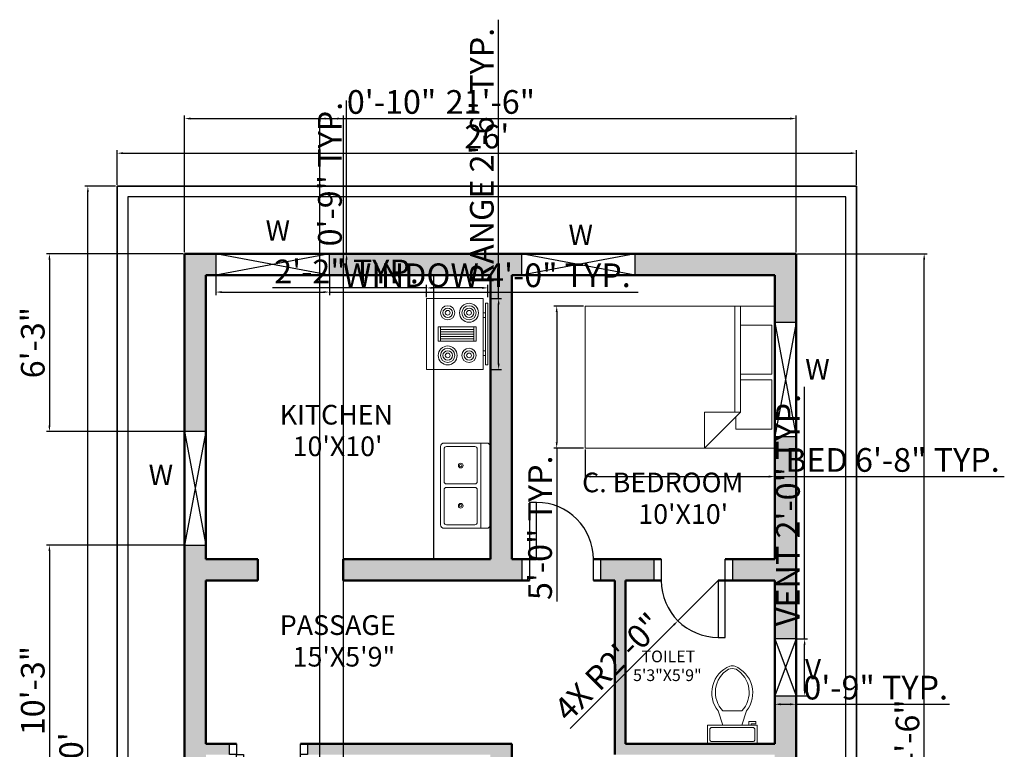
# Model space of a CAD drawing. Units: inches. Extents: x 2789 to 3623, y 2388 to 2993.
# Tile 2 of 5: x 2789 to 3205, y 2685 to 2993. Entities that reach past the tile are written whole.
import ezdxf

# ---------------------------------------------------------------- set-up
doc = ezdxf.new("R2010")
doc.units = ezdxf.units.IN
for name, color, linetype, lineweight in [('A-ANNO-DIMS', 2, 'Continuous', 18), ('A-ANNO-TEXT', 7, 'Continuous', 18), ('A-AREA-IDEN', 7, 'Continuous', 18), ('A-EQPM', 9, 'Continuous', 18), ('A-FLOR-CASE', 8, 'Continuous', 25), ('A-FLOR-FIXT', 9, 'Continuous', 18), ('A-FURN', 8, 'Continuous', 18), ('A-WALL', 7, 'Continuous', 50), ('A-WALL-PATT', 5, 'Continuous', 13), ('C-PROP', 7, 'Continuous', 35), ('d', 1, 'Continuous', 25), ('L-WALL', 7, 'Continuous', 25), ('v', 6, 'Continuous', 25), ('w', 170, 'Continuous', 25)]:
    doc.layers.add(name, color=color, linetype=linetype, lineweight=lineweight)
doc.styles.get("Standard").update_dxf_attribs({"font": 'arial.ttf'})
doc.dimstyles.new('ISO-25', dxfattribs={"dimtxt": 10, "dimasz": 2.5, "dimexe": 1.25, "dimexo": 0.625, "dimtad": 1, "dimlunit": 4, "dimtxsty": 'Standard', "dimcen": 2.5, "dimadec": 0, "dimazin": 0, "dimtfac": 1, "dimtmove": 0, "dimatfit": 3, "dimfxl": 1, "dimarcsym": 0})

# ---------------------------------------------------------------- blocks, each defined once
blk = doc.blocks.new('Range-Oven - 30 in top')
for p, q in [((0, -3), (30, -3)), ((12, -6), (18, -6)), ((13, -20), (13, -6)), ((14, -6), (14, -20)), ((15, -20), (15, -6)), ((16, -6), (16, -20)), ((17, -20), (17, -6)), ((18, -20), (12, -20)), ((6, -24), (6, -25)), ((8, -25), (8, -24)), ((22, -25), (22, -24)), ((24, -24), (24, -25))]:
    blk.add_line(p, q)
for points in [[(0, -24), (0, 0), (30, 0), (30, -24)], [(12, -21), (12, -5), (18, -5), (18, -21)], [(2, -26), (2, -25), (28, -25), (28, -26)]]:
    blk.add_lwpolyline(points, close=True)
for centre, radius in [((6, -9), 4), ((6, -9), 3), ((6, -9), 2), ((6, -9), 1), ((24, -9), 3), ((24, -9), 2), ((24, -9), 1), ((6, -18), 3), ((6, -18), 2), ((24, -18), 4), ((24, -18), 3), ((24, -18), 2), ((6, -18), 1), ((24, -18), 1)]:
    blk.add_circle(centre, radius)
blk = doc.blocks.new('Sink-double - 36 in top')
for p, q in [((-18, -4), (18, -4)), ((-0.75, -18.5), (-0.75, -6.5)), ((0.75, -6.5), (0.75, -18.5))]:
    blk.add_line(p, q)
for points in [[(-16.5, 0), (16.5, 0)], [(-18, -19.5), (-18, -1.5)], [(18, -1.5), (18, -19.5)], [(-16.5, -18.5), (-16.5, -6.5)], [(-15.5, -5.5), (-1.75, -5.5)], [(1.75, -5.5), (15.5, -5.5)], [(16.5, -6.5), (16.5, -18.5)], [(-1.75, -19.5), (-15.5, -19.5)], [(15.5, -19.5), (1.75, -19.5)], [(16.5, -21), (-16.5, -21)]]:
    blk.add_lwpolyline(points)
for centre, radius in [((-8.5, -12.5), 1), ((-8.5, -12.5), 0.5), ((8.5, -12.5), 1), ((8.5, -12.5), 0.5)]:
    blk.add_circle(centre, radius)
for centre, radius, start, end in [((-16.5, -1.5), 1.5, 90, 180), ((16.5, -1.5), 1.5, 0, 90), ((-15.5, -6.5), 1, 90, 180), ((-1.75, -6.5), 1, 0, 90), ((1.75, -6.5), 1, 90, 180), ((15.5, -6.5), 1, 0, 90), ((-16.5, -19.5), 1.5, 180, 270), ((-15.5, -18.5), 1, 180, 270), ((-1.75, -18.5), 1, 270, 0), ((1.75, -18.5), 1, 180, 270), ((15.5, -18.5), 1, 270, 0), ((16.5, -19.5), 1.5, 270, 0)]:
    blk.add_arc(centre, radius, start, end)
blk = doc.blocks.new('Toilet - top')
for p, q in [((9.5, -6), (9.5, -2)), ((-8, -8.5), (-8, -8)), ((-7, -8), (-7, -9.5)), ((-4, -8), (-6, -14)), ((4, -8), (6, -14)), ((-10, -8.5), (-8, -8.5)), ((-10, -9.5), (-10, -8.5)), ((-7, -9.5), (-10, -9.5)), ((4, -14), (-4, -14))]:
    blk.add_line(p, q)
blk.add_lwpolyline([(10.5, -8), (10.5, 0), (-10.5, 0), (-10.5, -8)], close=True)
for points in [[(-9.5, -2), (-9.5, -6)], [(8.5, -1), (-8.5, -1)], [(-8.5, -7), (8.5, -7)]]:
    blk.add_lwpolyline(points)
for centre, radius, start, end in [((-8.62, -1.88), 0.884, 81.8699, 188.1301), ((8.62, -1.88), 0.884, 351.8699, 98.1301), ((-8.62, -6.12), 0.884, 171.8699, 278.1301), ((8.62, -6.12), 0.884, 261.8699, 8.1301), ((3.52, -21.58), 12.17, 141.4691, 247.9714), ((4.2, -21.82), 11.33, 136.3677, 238.9468), ((-3.52, -21.58), 12.17, 292.0284, 38.5307), ((-4.2, -21.82), 11.33, 301.053, 43.6321), ((0, -27.88), 4, 245.7318, 294.2682), ((0, -29), 4, 254.8605, 285.1395)]:
    blk.add_arc(centre, radius, start, end)
blk = doc.blocks.new('Bed - Queen')
for p, q in [((0, -80.00003), (0, 0)), ((0, 0), (59.99999, 0)), ((59.99999, 0), (59.99999, -80.00003)), ((7.99999, -1.2), (28.79998, -1.2)), ((7.99999, -14.4), (7.99999, -1.2)), ((28.79998, -1.2), (28.79998, -14.4)), ((31.19999, -1.2), (51.99999, -1.2)), ((31.19999, -14.4), (31.19999, -1.2)), ((51.99999, -1.2), (51.99999, -16.4)), ((0, -14.4), (44.8, -14.4)), ((59.99999, -29.6), (44.8, -14.4)), ((44.8, -14.4), (44.8, -29.6)), ((51.99999, -16.4), (46.79936, -16.4)), ((44.8, -16.8), (0, -16.8)), ((44.8, -29.6), (59.99999, -29.6)), ((59.99999, -80.00003), (0, -80.00003))]:
    blk.add_line(p, q)
blk = doc.blocks.new('*D12')
at = {"layer": 'A-ANNO-DIMS', "color": 0, "lineweight": -2, "transparency": 16777216}
for p, q in [((2830.55, 2923.47), (2830.55, 2938.03)), ((3142.55, 2923.47), (3142.55, 2938.03)), ((2833.05, 2936.78), (3140.05, 2936.78))]:
    blk.add_line(p, q, dxfattribs=at)
at = {"layer": 'A-ANNO-DIMS', "color": 0, "transparency": 16777216}
for points in [[(2833.05, 2937.19), (2833.05, 2936.36), (2830.55, 2936.78)], [(3140.05, 2937.19), (3140.05, 2936.36), (3142.55, 2936.78)]]:
    blk.add_solid(points, dxfattribs=at)
at = {"layer": 'Defpoints', "color": 0, "transparency": 16777216}
for p in [(3142.55, 2936.78), (2830.55, 2922.84), (3142.55, 2922.84)]:
    blk.add_point(p, dxfattribs=at)
at = {"layer": 'A-ANNO-DIMS', "color": 0, "transparency": 16777216, "insert": (2986.55, 2942.51), "char_height": 10, "attachment_point": 5}
blk.add_mtext("26'", dxfattribs=at)
blk = doc.blocks.new('*D13')
at = {"layer": 'A-ANNO-DIMS', "color": 0, "lineweight": -2, "transparency": 16777216}
for p, q in [((2829.92, 2922.84), (2816.96, 2922.84)), ((2818.21, 2445.34), (2818.21, 2920.34)), ((2829.92, 2442.84), (2816.96, 2442.84))]:
    blk.add_line(p, q, dxfattribs=at)
at = {"layer": 'A-ANNO-DIMS', "color": 0, "transparency": 16777216}
for points in [[(2817.8, 2920.34), (2818.63, 2920.34), (2818.21, 2922.84)], [(2817.8, 2445.34), (2818.63, 2445.34), (2818.21, 2442.84)]]:
    blk.add_solid(points, dxfattribs=at)
at = {"layer": 'Defpoints', "color": 0, "transparency": 16777216}
for p in [(2818.21, 2922.84), (2830.55, 2922.84), (2830.55, 2442.84)]:
    blk.add_point(p, dxfattribs=at)
at = {"layer": 'A-ANNO-DIMS', "color": 0, "transparency": 16777216, "insert": (2812.48, 2682.84), "char_height": 10, "attachment_point": 5, "rotation": 90}
blk.add_mtext("40'", dxfattribs=at)
blk = doc.blocks.new('DOOR-24IN-JAMB-9IN')
for points in [[(0, 24), (-3, 24), (-3, 0), (0, 0)], [(-6, 0), (-3, 0), (-3, -9), (-6, -9)], [(24, 0), (27, 0), (27, -9), (24, -9)]]:
    blk.add_lwpolyline(points, close=True)
blk.add_arc((0, 0), 24, 0, 90)
blk = doc.blocks.new('DOOR-24IN-JAMB-4_5IN')
for points in [[(-3, 0), (-6, 0), (-6, 4.5), (-3, 4.5)], [(27, 0), (24, 0), (24, 4.5), (27, 4.5)], [(0, -24), (-3, -24), (-3, 0), (0, 0)]]:
    blk.add_lwpolyline(points, close=True)
blk.add_arc((0, 0), 24, 270, 0)
blk = doc.blocks.new('WINDOW-48IN')
for p, q in [((48, 9), (0, 0)), ((48, 0), (0, 9))]:
    blk.add_line(p, q)
blk.add_lwpolyline([(0, 9), (0, 0), (48, 0), (48, 9)], close=True)
blk = doc.blocks.new('VENT-24IN')
for p, q in [((0, 24), (9, 0)), ((9, 24), (0, 0))]:
    blk.add_line(p, q)
blk.add_lwpolyline([(0, 0), (9, 0), (9, 24), (0, 24)], close=True)
blk = doc.blocks.new('*D20')
at = {"layer": 'A-ANNO-DIMS', "color": 0, "lineweight": -2, "transparency": 16777216}
for p, q in [((2872.18, 2884.72), (2872.18, 2876.89)), ((2920.18, 2884.72), (2920.18, 2876.89)), ((2874.68, 2878.14), (2917.68, 2878.14)), ((2920.18, 2878.14), (3050.48, 2878.14))]:
    blk.add_line(p, q, dxfattribs=at)
at = {"layer": 'A-ANNO-DIMS', "color": 0, "transparency": 16777216}
for points in [[(2874.68, 2878.56), (2874.68, 2877.73), (2872.18, 2878.14)], [(2917.68, 2878.56), (2917.68, 2877.73), (2920.18, 2878.14)]]:
    blk.add_solid(points, dxfattribs=at)
at = {"layer": 'Defpoints', "color": 0, "transparency": 16777216}
for p in [(2872.18, 2885.34), (2920.18, 2885.34), (2920.18, 2878.14)]:
    blk.add_point(p, dxfattribs=at)
at = {"layer": 'A-ANNO-DIMS', "color": 0, "transparency": 16777216, "insert": (2986.58, 2883.94), "char_height": 10, "attachment_point": 5}
blk.add_mtext('WINDOW 4\'-0" TYP.', dxfattribs=at)
blk = doc.blocks.new('*D21')
at = {"layer": 'A-ANNO-DIMS', "color": 0, "lineweight": -2, "transparency": 16777216}
for p, q in [((2927.38, 2894.34), (2927.38, 2959.05)), ((2920.81, 2894.34), (2928.63, 2894.34)), ((2927.38, 2887.84), (2927.38, 2891.84)), ((2920.81, 2885.34), (2928.63, 2885.34))]:
    blk.add_line(p, q, dxfattribs=at)
at = {"layer": 'A-ANNO-DIMS', "color": 0, "transparency": 16777216}
for points in [[(2926.97, 2891.84), (2927.8, 2891.84), (2927.38, 2894.34)], [(2926.97, 2887.84), (2927.8, 2887.84), (2927.38, 2885.34)]]:
    blk.add_solid(points, dxfattribs=at)
at = {"layer": 'Defpoints', "color": 0, "transparency": 16777216}
for p in [(2920.18, 2894.34), (2927.38, 2894.34), (2920.18, 2885.34)]:
    blk.add_point(p, dxfattribs=at)
at = {"layer": 'A-ANNO-DIMS', "color": 0, "transparency": 16777216, "insert": (2921.65, 2927.94), "char_height": 10, "attachment_point": 5, "rotation": 90}
blk.add_mtext('0\'-9" TYP.', dxfattribs=at)
blk = doc.blocks.new('*D24')
at = {"layer": 'A-ANNO-DIMS', "color": 0, "lineweight": -2, "transparency": 16777216}
for p, q in [((3028.05, 2811.61), (3028.05, 2798.99)), ((3108.05, 2811.61), (3108.05, 2798.99)), ((3030.55, 2800.24), (3105.55, 2800.24)), ((3108.05, 2800.24), (3204.92, 2800.24))]:
    blk.add_line(p, q, dxfattribs=at)
at = {"layer": 'A-ANNO-DIMS', "color": 0, "transparency": 16777216}
for points in [[(3030.55, 2800.66), (3030.55, 2799.82), (3028.05, 2800.24)], [(3105.55, 2800.66), (3105.55, 2799.82), (3108.05, 2800.24)]]:
    blk.add_solid(points, dxfattribs=at)
at = {"layer": 'Defpoints', "color": 0, "transparency": 16777216}
for p in [(3028.05, 2812.24), (3108.05, 2812.24), (3108.05, 2800.24)]:
    blk.add_point(p, dxfattribs=at)
at = {"layer": 'A-ANNO-DIMS', "color": 0, "transparency": 16777216, "insert": (3157.73, 2805.97), "char_height": 10, "attachment_point": 5}
blk.add_mtext('BED 6\'-8" TYP.', dxfattribs=at)
blk = doc.blocks.new('*D25')
at = {"layer": 'A-ANNO-DIMS', "color": 0, "lineweight": -2, "transparency": 16777216}
for p, q in [((3027.42, 2872.24), (3014.8, 2872.24)), ((3016.05, 2869.74), (3016.05, 2814.74)), ((3027.42, 2812.24), (3014.8, 2812.24)), ((3016.05, 2812.24), (3016.05, 2747.53))]:
    blk.add_line(p, q, dxfattribs=at)
at = {"layer": 'A-ANNO-DIMS', "color": 0, "transparency": 16777216}
for points in [[(3015.63, 2869.74), (3016.46, 2869.74), (3016.05, 2872.24)], [(3015.63, 2814.74), (3016.46, 2814.74), (3016.05, 2812.24)]]:
    blk.add_solid(points, dxfattribs=at)
at = {"layer": 'Defpoints', "color": 0, "transparency": 16777216}
for p in [(3028.05, 2872.24), (3016.05, 2812.24), (3028.05, 2812.24)]:
    blk.add_point(p, dxfattribs=at)
at = {"layer": 'A-ANNO-DIMS', "color": 0, "transparency": 16777216, "insert": (3010.32, 2778.64), "char_height": 10, "attachment_point": 5, "rotation": 90}
blk.add_mtext('5\'-0" TYP.', dxfattribs=at)
blk = doc.blocks.new('*D28')
at = {"layer": 'A-ANNO-DIMS', "color": 0, "lineweight": -2, "transparency": 16777216}
for p, q in [((2991.55, 2875.4), (2991.55, 2993.15)), ((2987.67, 2875.4), (2992.8, 2875.4)), ((2991.55, 2847.9), (2991.55, 2872.9)), ((2987.67, 2845.4), (2992.8, 2845.4))]:
    blk.add_line(p, q, dxfattribs=at)
at = {"layer": 'A-ANNO-DIMS', "color": 0, "transparency": 16777216}
for points in [[(2991.13, 2872.9), (2991.96, 2872.9), (2991.55, 2875.4)], [(2991.13, 2847.9), (2991.96, 2847.9), (2991.55, 2845.4)]]:
    blk.add_solid(points, dxfattribs=at)
at = {"layer": 'Defpoints', "color": 0, "transparency": 16777216}
for p in [(2987.05, 2875.4), (2991.55, 2875.4), (2987.05, 2845.4)]:
    blk.add_point(p, dxfattribs=at)
at = {"layer": 'A-ANNO-DIMS', "color": 0, "transparency": 16777216, "insert": (2985.75, 2935.53), "char_height": 10, "attachment_point": 5, "rotation": 90}
blk.add_mtext('RANGE 2\'-6" TYP.', dxfattribs=at)
blk = doc.blocks.new('*D29')
at = {"layer": 'A-ANNO-DIMS', "color": 0, "lineweight": -2, "transparency": 16777216}
for p, q in [((2961.05, 2879.9), (2896.17, 2879.9)), ((2961.05, 2876.03), (2961.05, 2881.15)), ((2984.55, 2879.9), (2963.55, 2879.9)), ((2987.05, 2876.03), (2987.05, 2881.15))]:
    blk.add_line(p, q, dxfattribs=at)
at = {"layer": 'A-ANNO-DIMS', "color": 0, "transparency": 16777216}
for points in [[(2963.55, 2880.32), (2963.55, 2879.49), (2961.05, 2879.9)], [(2984.55, 2880.32), (2984.55, 2879.49), (2987.05, 2879.9)]]:
    blk.add_solid(points, dxfattribs=at)
at = {"layer": 'Defpoints', "color": 0, "transparency": 16777216}
for p in [(2961.05, 2879.9), (2961.05, 2875.4), (2987.05, 2875.4)]:
    blk.add_point(p, dxfattribs=at)
at = {"layer": 'A-ANNO-DIMS', "color": 0, "transparency": 16777216, "insert": (2927.36, 2885.55), "char_height": 10, "attachment_point": 5}
blk.add_mtext('2\'-2" TYP.', dxfattribs=at)
blk = doc.blocks.new('*D40')
at = {"layer": 'A-ANNO-DIMS', "color": 0, "lineweight": -2, "transparency": 16777216}
for p, q in [((3120.65, 2731.71), (3120.65, 2838.07)), ((3117.67, 2731.71), (3121.9, 2731.71)), ((3120.65, 2710.21), (3120.65, 2729.21)), ((3117.67, 2707.71), (3121.9, 2707.71))]:
    blk.add_line(p, q, dxfattribs=at)
at = {"layer": 'A-ANNO-DIMS', "color": 0, "transparency": 16777216}
for points in [[(3120.23, 2729.21), (3121.06, 2729.21), (3120.65, 2731.71)], [(3120.23, 2710.21), (3121.06, 2710.21), (3120.65, 2707.71)]]:
    blk.add_solid(points, dxfattribs=at)
at = {"layer": 'Defpoints', "color": 0, "transparency": 16777216}
for p in [(3117.05, 2731.71), (3120.65, 2731.71), (3117.05, 2707.71)]:
    blk.add_point(p, dxfattribs=at)
at = {"layer": 'A-ANNO-DIMS', "color": 0, "transparency": 16777216, "insert": (3114.92, 2786.14), "char_height": 10, "attachment_point": 5, "rotation": 90}
blk.add_mtext('VENT 2\'-0" TYP.', dxfattribs=at)
blk = doc.blocks.new('*D41')
at = {"layer": 'A-ANNO-DIMS', "color": 0, "lineweight": -2, "transparency": 16777216}
for p, q in [((3108.05, 2707.09), (3108.05, 2702.86)), ((3117.05, 2707.09), (3117.05, 2702.86)), ((3110.55, 2704.11), (3114.55, 2704.11)), ((3117.05, 2704.11), (3181.75, 2704.11))]:
    blk.add_line(p, q, dxfattribs=at)
at = {"layer": 'A-ANNO-DIMS', "color": 0, "transparency": 16777216}
for points in [[(3110.55, 2704.53), (3110.55, 2703.69), (3108.05, 2704.11)], [(3114.55, 2704.53), (3114.55, 2703.69), (3117.05, 2704.11)]]:
    blk.add_solid(points, dxfattribs=at)
at = {"layer": 'Defpoints', "color": 0, "transparency": 16777216}
for p in [(3108.05, 2707.71), (3117.05, 2707.71), (3117.05, 2704.11)]:
    blk.add_point(p, dxfattribs=at)
at = {"layer": 'A-ANNO-DIMS', "color": 0, "transparency": 16777216, "insert": (3150.65, 2709.84), "char_height": 10, "attachment_point": 5}
blk.add_mtext('0\'-9" TYP.', dxfattribs=at)
blk = doc.blocks.new('*D42')
at = {"layer": 'A-ANNO-DIMS', "color": 0, "lineweight": -2, "transparency": 16777216}
for p, q in [((2859.05, 2894.97), (2859.05, 2952.64)), ((2861.55, 2951.39), (3114.55, 2951.39)), ((3117.05, 2894.97), (3117.05, 2952.64))]:
    blk.add_line(p, q, dxfattribs=at)
at = {"layer": 'A-ANNO-DIMS', "color": 0, "transparency": 16777216}
for points in [[(2861.55, 2951.81), (2861.55, 2950.98), (2859.05, 2951.39)], [(3114.55, 2951.81), (3114.55, 2950.98), (3117.05, 2951.39)]]:
    blk.add_solid(points, dxfattribs=at)
at = {"layer": 'Defpoints', "color": 0, "transparency": 16777216}
for p in [(3117.05, 2951.39), (2859.05, 2894.34), (3117.05, 2894.34)]:
    blk.add_point(p, dxfattribs=at)
at = {"layer": 'A-ANNO-DIMS', "color": 0, "transparency": 16777216, "insert": (2988.05, 2957.12), "char_height": 10, "attachment_point": 5}
blk.add_mtext('21\'-6"', dxfattribs=at)
blk = doc.blocks.new('*D43')
at = {"layer": 'A-ANNO-DIMS', "color": 0, "lineweight": -2, "transparency": 16777216}
for p, q in [((3117.67, 2894.34), (3172.35, 2894.34)), ((3171.1, 2482.84), (3171.1, 2891.84)), ((3117.67, 2480.34), (3172.35, 2480.34))]:
    blk.add_line(p, q, dxfattribs=at)
at = {"layer": 'A-ANNO-DIMS', "color": 0, "transparency": 16777216}
for points in [[(3170.68, 2891.84), (3171.51, 2891.84), (3171.1, 2894.34)], [(3170.68, 2482.84), (3171.51, 2482.84), (3171.1, 2480.34)]]:
    blk.add_solid(points, dxfattribs=at)
at = {"layer": 'Defpoints', "color": 0, "transparency": 16777216}
for p in [(3117.05, 2894.34), (3171.1, 2894.34), (3117.05, 2480.34)]:
    blk.add_point(p, dxfattribs=at)
at = {"layer": 'A-ANNO-DIMS', "color": 0, "transparency": 16777216, "insert": (3165.36, 2687.34), "char_height": 10, "attachment_point": 5, "rotation": 90}
blk.add_mtext('34\'-6"', dxfattribs=at)
blk = doc.blocks.new('*D48')
at = {"layer": 'A-ANNO-DIMS', "color": 0, "lineweight": -2, "transparency": 16777216}
for p, q in [((2916.05, 2520.72), (2916.05, 2952.64)), ((2918.55, 2951.39), (2923.55, 2951.39)), ((2926.05, 2520.72), (2926.05, 2952.64)), ((2926.05, 2951.39), (2964.15, 2951.39))]:
    blk.add_line(p, q, dxfattribs=at)
at = {"layer": 'A-ANNO-DIMS', "color": 0, "transparency": 16777216}
for points in [[(2918.55, 2951.81), (2918.55, 2950.98), (2916.05, 2951.39)], [(2923.55, 2951.81), (2923.55, 2950.98), (2926.05, 2951.39)]]:
    blk.add_solid(points, dxfattribs=at)
at = {"layer": 'Defpoints', "color": 0, "transparency": 16777216}
for p in [(2926.05, 2951.39), (2916.05, 2520.09), (2926.05, 2520.09)]:
    blk.add_point(p, dxfattribs=at)
at = {"layer": 'A-ANNO-DIMS', "color": 0, "transparency": 16777216, "insert": (2946.35, 2957.12), "char_height": 10, "attachment_point": 5}
blk.add_mtext('0\'-10"', dxfattribs=at)
blk = doc.blocks.new('*D52')
at = {"layer": 'A-ANNO-DIMS', "color": 0, "lineweight": -2, "transparency": 16777216}
for p, q in [((2858.42, 2894.34), (2800.75, 2894.34)), ((2802, 2891.84), (2802, 2821.77)), ((2858.42, 2819.27), (2800.75, 2819.27))]:
    blk.add_line(p, q, dxfattribs=at)
at = {"layer": 'A-ANNO-DIMS', "color": 0, "transparency": 16777216}
for points in [[(2801.58, 2891.84), (2802.41, 2891.84), (2802, 2894.34)], [(2801.58, 2821.77), (2802.41, 2821.77), (2802, 2819.27)]]:
    blk.add_solid(points, dxfattribs=at)
at = {"layer": 'Defpoints', "color": 0, "transparency": 16777216}
for p in [(2859.05, 2894.34), (2802, 2819.27), (2859.05, 2819.27)]:
    blk.add_point(p, dxfattribs=at)
at = {"layer": 'A-ANNO-DIMS', "color": 0, "transparency": 16777216, "insert": (2796.26, 2856.8), "char_height": 10, "attachment_point": 5, "rotation": 90}
blk.add_mtext('6\'-3"', dxfattribs=at)
blk = doc.blocks.new('*D53')
at = {"layer": 'A-ANNO-DIMS', "color": 0, "lineweight": -2, "transparency": 16777216}
for p, q in [((2858.42, 2771.27), (2800.75, 2771.27)), ((2802, 2768.77), (2802, 2651.02)), ((2858.42, 2648.52), (2800.75, 2648.52))]:
    blk.add_line(p, q, dxfattribs=at)
at = {"layer": 'A-ANNO-DIMS', "color": 0, "transparency": 16777216}
for points in [[(2801.58, 2768.77), (2802.41, 2768.77), (2802, 2771.27)], [(2801.58, 2651.02), (2802.41, 2651.02), (2802, 2648.52)]]:
    blk.add_solid(points, dxfattribs=at)
at = {"layer": 'Defpoints', "color": 0, "transparency": 16777216}
for p in [(2859.05, 2771.27), (2802, 2648.52), (2859.05, 2648.52)]:
    blk.add_point(p, dxfattribs=at)
at = {"layer": 'A-ANNO-DIMS', "color": 0, "transparency": 16777216, "insert": (2796.26, 2709.89), "char_height": 10, "attachment_point": 5, "rotation": 90}
blk.add_mtext('10\'-3"', dxfattribs=at)
blk = doc.blocks.new('*D59')
at = {"layer": 'A-ANNO-DIMS', "color": 0, "lineweight": -2, "transparency": 16777216}
for p, q in [((3084.18, 2756.34), (3067.21, 2739.37)), ((3021.75, 2693.91), (3065.44, 2737.6))]:
    blk.add_line(p, q, dxfattribs=at)
at = {"layer": 'A-ANNO-DIMS', "color": 0, "transparency": 16777216}
blk.add_solid([(3065.15, 2737.9), (3065.74, 2737.31), (3067.21, 2739.37)], dxfattribs=at)
at = {"layer": 'Defpoints', "color": 0, "transparency": 16777216}
for p in [(3084.18, 2756.34), (3067.21, 2739.37)]:
    blk.add_point(p, dxfattribs=at)
at = {"layer": 'A-ANNO-DIMS', "color": 0, "transparency": 16777216, "insert": (3038.66, 2718.92), "char_height": 10, "attachment_point": 5, "rotation": 45.0007}
blk.add_mtext('4X R2\'-0"', dxfattribs=at)

msp = doc.modelspace()

# ---------------------------------------------------------------- hatches: boundary and pattern name
at = {"layer": 'A-WALL-PATT'}
h = msp.add_hatch(color=256, dxfattribs=at)
h.dxf.hatch_style = 1
h.paths.add_polyline_path([(2868.048, 2600.516), (2859.048, 2600.516), (2859.048, 2480.342), (2996.048, 2480.342), (2996.048, 2489.342), (2868.048, 2489.342), (2868.048, 2553.842), (3004.548, 2553.842), (3004.548, 2562.842), (2997.048, 2562.842), (2997.048, 2687.342), (2910.917, 2687.342), (2910.917, 2682.842), (2988.048, 2682.842), (2988.048, 2562.842), (2868.048, 2562.842)])
h.paths.add_polyline_path([(2996.048, 2523.092), (2916.048, 2523.092), (2916.048, 2520.092), (2996.048, 2520.092)], flags=17)
h.paths.add_polyline_path([(3065.118, 2562.842), (3052.548, 2562.842), (3052.548, 2553.842), (3065.118, 2553.842)])
h.paths.add_polyline_path([(3117.048, 2569.319), (3108.048, 2569.319), (3108.048, 2562.842), (3098.118, 2562.842), (3098.118, 2553.842), (3117.048, 2553.842)])
h.paths.add_polyline_path([(3117.048, 2707.71), (3108.048, 2707.71), (3108.048, 2687.342), (3045.048, 2687.342), (3045.048, 2756.342), (3057.181, 2756.342), (3057.181, 2765.342), (3034.539, 2765.342), (3034.539, 2756.342), (3040.548, 2756.342), (3040.548, 2682.842), (3108.048, 2682.842), (3108.048, 2617.319), (3117.048, 2617.319)])
h.paths.add_polyline_path([(3117.048, 2817.229), (3108.048, 2817.229), (3108.048, 2812.239), (3108.048, 2765.342), (3090.181, 2765.342), (3090.181, 2756.342), (3108.048, 2756.342), (3108.048, 2731.71), (3117.048, 2731.71)])
h.paths.add_polyline_path([(2868.048, 2682.842), (2877.917, 2682.842), (2877.917, 2687.342), (2868.048, 2687.342), (2868.048, 2756.342), (2889.977, 2756.342), (2889.977, 2765.342), (2868.048, 2765.342), (2868.048, 2771.267), (2859.048, 2771.267), (2859.048, 2648.516), (2868.048, 2648.516)])
h.paths.add_polyline_path([(3001.539, 2765.342), (2997.048, 2765.342), (2997.048, 2885.342), (3001.182, 2885.342), (3001.182, 2894.342), (2920.184, 2894.342), (2920.184, 2885.342), (2988.048, 2885.342), (2988.048, 2765.342), (2925.977, 2765.342), (2925.977, 2756.342), (3001.539, 2756.342)])
h.paths.add_polyline_path([(2868.048, 2885.342), (2872.184, 2885.342), (2872.184, 2894.342), (2859.048, 2894.342), (2859.048, 2819.267), (2868.048, 2819.267)])
h.paths.add_polyline_path([(3117.048, 2894.342), (3049.182, 2894.342), (3049.182, 2885.342), (3108.048, 2885.342), (3108.048, 2865.229), (3117.048, 2865.229)])
h.paths.add_polyline_path([(3025.421, 2540.366), (3041.067, 2540.366), (3041.067, 2553.271), (3025.421, 2553.271)], flags=9)
h.paths.add_polyline_path([(3118.771, 2839.078), (3134.416, 2839.078), (3134.416, 2851.983), (3118.771, 2851.983)], flags=9)
h.paths.add_polyline_path([(3118.682, 2712.44), (3131, 2712.44), (3131, 2725.345), (3118.682, 2725.345)], flags=9)
h.paths.add_polyline_path([(3118.47, 2582.859), (3134.115, 2582.859), (3134.115, 2595.763), (3118.47, 2595.763)], flags=9)
h.paths.add_polyline_path([(2842.843, 2619.924), (2858.489, 2619.924), (2858.489, 2632.829), (2842.843, 2632.829)], flags=9)
h.paths.add_polyline_path([(2841.723, 2794.475), (2857.368, 2794.475), (2857.368, 2807.38), (2841.723, 2807.38)], flags=9)
h.paths.add_polyline_path([(3018.872, 2895.803), (3034.517, 2895.803), (3034.517, 2908.708), (3018.872, 2908.708)], flags=9)
h.paths.add_polyline_path([(2891.065, 2897.701), (2906.71, 2897.701), (2906.71, 2910.606), (2891.065, 2910.606)], flags=9)
h.paths.add_polyline_path([(2898.76, 2503.274), (2898.76, 2543.14), (2886.045, 2543.14), (2886.045, 2503.274)], flags=25)
h.paths.add_polyline_path([(2885.453, 2497.829), (2885.453, 2542.718), (2872.568, 2542.718), (2872.568, 2497.829)], flags=25)
h.paths.add_polyline_path([(3033.853, 2492.441), (3086.618, 2492.441), (3086.618, 2505.156), (3033.853, 2505.156)], flags=9)
h.paths.add_polyline_path([(3039.46, 2505.748), (3086.274, 2505.748), (3086.274, 2518.633), (3039.46, 2518.633)], flags=9)
h.paths.add_polyline_path([(3048.345, 2778.023), (3090.544, 2778.023), (3090.544, 2790.738), (3048.345, 2790.738)], flags=9)
h.paths.add_polyline_path([(3024.618, 2791.33), (3106.873, 2791.33), (3106.873, 2804.214), (3024.618, 2804.214)], flags=9)
h.paths.add_polyline_path([(3047.007, 2712.567), (3076.988, 2712.567), (3076.988, 2720.13), (3047.007, 2720.13)], flags=25)
h.paths.add_polyline_path([(3050.563, 2720.481), (3079.162, 2720.481), (3079.162, 2728.14), (3050.563, 2728.14)], flags=25)
h.paths.add_polyline_path([(3000.345, 2609.496), (3042.544, 2609.496), (3042.544, 2622.211), (3000.345, 2622.211)], flags=9)
h.paths.add_polyline_path([(3001.972, 2623.016), (3035.131, 2623.016), (3035.131, 2635.468), (3001.972, 2635.468)], flags=9)
h.paths.add_polyline_path([(2910.315, 2645.374), (2952.514, 2645.374), (2952.514, 2658.089), (2910.315, 2658.089)], flags=25)
h.paths.add_polyline_path([(2904.87, 2658.68), (2985.189, 2658.68), (2985.189, 2671.565), (2904.87, 2671.565)], flags=25)
h.paths.add_polyline_path([(2902.494, 2717.778), (2948.81, 2717.778), (2948.81, 2730.493), (2902.494, 2730.493)], flags=9)
h.paths.add_polyline_path([(2897.051, 2731.086), (2956.772, 2731.086), (2956.772, 2743.962), (2897.051, 2743.962)], flags=9)
h.paths.add_polyline_path([(2902.494, 2806.621), (2944.693, 2806.621), (2944.693, 2819.336), (2902.494, 2819.336)], flags=9)
h.paths.add_polyline_path([(2897.051, 2819.929), (2955.464, 2819.929), (2955.464, 2832.806), (2897.051, 2832.806)], flags=9)

# ---------------------------------------------------------------- linework, layer by layer
at = {"layer": 'A-FLOR-CASE'}
msp.add_line((2964.048, 2885.342), (2964.048, 2765.342), dxfattribs=at)
at = {"layer": 'A-WALL'}
for p, q in [((2859.048, 2894.342), (2859.048, 2480.342)), ((3117.048, 2894.342), (2859.048, 2894.342)), ((3117.048, 2553.842), (3117.048, 2894.342)), ((2868.048, 2885.342), (2868.048, 2765.342)), ((2988.048, 2885.342), (2868.048, 2885.342)), ((2988.048, 2885.342), (2988.048, 2765.342)), ((3108.048, 2885.342), (2997.048, 2885.342)), ((2997.048, 2885.342), (2997.048, 2765.342)), ((3108.048, 2765.342), (3108.048, 2885.342)), ((2889.977, 2765.342), (2868.048, 2765.342)), ((2889.977, 2756.342), (2889.977, 2765.342)), ((2988.048, 2765.342), (2925.977, 2765.342)), ((2925.977, 2756.342), (2925.977, 2765.342)), ((3007.539, 2765.342), (2997.048, 2765.342)), ((3060.181, 2765.342), (3031.539, 2765.342)), ((3108.048, 2765.342), (3087.181, 2765.342)), ((2868.048, 2756.342), (2868.048, 2687.342)), ((2889.977, 2756.342), (2868.048, 2756.342)), ((3004.539, 2756.342), (2925.977, 2756.342)), ((3040.548, 2756.342), (3031.539, 2756.342)), ((3040.548, 2682.842), (3040.548, 2756.342)), ((3045.048, 2687.342), (3045.048, 2756.342)), ((3060.181, 2756.342), (3045.048, 2756.342)), ((3108.048, 2756.342), (3084.181, 2756.342)), ((3108.048, 2687.342), (3108.048, 2756.342)), ((2880.917, 2687.342), (2868.048, 2687.342)), ((2997.048, 2687.342), (2907.917, 2687.342)), ((2997.048, 2687.342), (2997.048, 2562.842)), ((3108.048, 2687.342), (3045.048, 2687.342))]:
    msp.add_line(p, q, dxfattribs=at)
at = {"layer": 'C-PROP'}
msp.add_lwpolyline([(2830.548, 2442.842), (3142.548, 2442.842), (3142.548, 2922.842), (2830.548, 2922.842)], close=True, dxfattribs=at)
at = {"layer": 'L-WALL'}
for p, q in [((3138.048, 2918.342), (2835.048, 2918.342)), ((2835.048, 2918.342), (2835.048, 2447.342)), ((3138.048, 2447.342), (3138.048, 2918.342))]:
    msp.add_line(p, q, dxfattribs=at)

# ---------------------------------------------------------------- block references
at = {"layer": 'A-EQPM', "rotation": 90}
msp.add_blockref('Range-Oven - 30 in top', (2961.048, 2845.404), dxfattribs=at)
at = {"layer": 'A-FLOR-FIXT'}
for name, p, rotation in [('Sink-double - 36 in top', (2988.048, 2796.411), 270), ('Toilet - top', (3090.13, 2687.342), 180)]:
    msp.add_blockref(name, p, dxfattribs=dict(at, rotation=rotation))
at = {"layer": 'A-FURN', "rotation": 270}
msp.add_blockref('Bed - Queen', (3108.048, 2872.239), dxfattribs=at)
at = {"layer": 'd'}
for name, p in [('DOOR-24IN-JAMB-9IN', (3007.539, 2765.342)), ('DOOR-24IN-JAMB-4_5IN', (2883.917, 2682.842))]:
    msp.add_blockref(name, p, dxfattribs=at)
at = {"layer": 'd', "rotation": 180}
msp.add_blockref('DOOR-24IN-JAMB-9IN', (3084.181, 2756.342), dxfattribs=at)
at = {"layer": 'v'}
msp.add_blockref('VENT-24IN', (3108.048, 2707.71), dxfattribs=at)
at = {"layer": 'w'}
for p in [(2872.184, 2885.342), (3001.182, 2885.342)]:
    msp.add_blockref('WINDOW-48IN', p, dxfattribs=at)
at = {"layer": 'w', "rotation": 90.00000000000036}
for p in [(3117.048, 2817.229), (2868.048, 2771.267)]:
    msp.add_blockref('WINDOW-48IN', p, dxfattribs=at)

# ---------------------------------------------------------------- texts
at = {"layer": 'A-ANNO-TEXT'}
for s, p in [('W', (2893.216, 2899.852)), ('W', (3021.023, 2897.954)), ('W', (3120.922, 2841.229)), ('W', (2843.874, 2796.626)), ('V', (3120.833, 2714.591))]:
    msp.add_text(s, height=8.603, dxfattribs=at).set_placement(p)
at = {"layer": 'A-AREA-IDEN'}
for s, height, p in [('KITCHEN ', 8.3011, (2899.197, 2822.217)), ("10'X10'", 8.3011, (2904.613, 2808.882)), ('C. BEDROOM ', 8.30108, (3026.765, 2793.619)), ("10'X10'", 8.3011, (3050.465, 2780.284)), ('PASSAGE', 8.3011, (2899.197, 2733.374)), ('15\'X5\'9"', 8.3011, (2904.613, 2720.039)), ('TOILET ', 4.9345, (3051.839, 2721.842)), ('5\'3"X5\'9"', 4.9345, (3048.268, 2713.915))]:
    msp.add_text(s, height=height, dxfattribs=at).set_placement(p)

# ---------------------------------------------------------------- dimensions: what is measured, and where the dimension line sits
at = {"layer": 'A-ANNO-DIMS'}
for base, p1, p2, angle, text, picture, middle in [((2991.548, 2875.404), (2987.048, 2845.404), (2987.048, 2875.404), 90, 'RANGE <> TYP.', '*D28', (2985.753, 2935.527)), ((2927.384, 2894.342), (2920.184, 2885.342), (2920.184, 2894.342), 90, '<> TYP.', '*D21', (2921.653, 2927.944)), ((2961.048, 2879.904), (2987.048, 2875.404), (2961.048, 2875.404), 180, '<> TYP.', '*D29', (2927.36, 2885.553)), ((3016.048, 2812.239), (3028.048, 2872.239), (3028.048, 2812.239), 270, '<> TYP.', '*D25', (3010.317, 2778.637)), ((3120.648, 2731.71), (3117.048, 2707.71), (3117.048, 2731.71), 90, 'VENT <> TYP.', '*D40', (3114.917, 2786.142))]:
    dim = msp.add_linear_dim(base=base, p1=p1, p2=p2, angle=angle, text=text, dimstyle='ISO-25', override={"dimdec": 1, "dimlfac": 1, "dimrnd": 0, "dimzin": 1, "dimdsep": 46, "dimlunit": 4, "dimfrac": 2}, dxfattribs=at)
    dim.commit()
    dim.dimension.update_dxf_attribs({"geometry": picture, "text_midpoint": middle})
for base, p1, p2, override, picture, middle in [((3117.048, 2951.392), (2859.048, 2894.342), (3117.048, 2894.342), {"dimdec": 1, "dimlfac": 1, "dimrnd": 0, "dimzin": 1, "dimdsep": 46, "dimlunit": 4, "dimfrac": 2}, '*D42', (2988.048, 2957.122)), ((2926.048, 2951.392), (2916.048, 2520.092), (2926.048, 2520.092), {"dimdec": 1, "dimlfac": 1, "dimrnd": 0, "dimzin": 1, "dimdsep": 46, "dimlunit": 4, "dimfrac": 2}, '*D48', (2946.349, 2957.122)), ((3142.548, 2936.777), (2830.548, 2922.842), (3142.548, 2922.842), {"dimclrd": 0, "dimclre": 0, "dimclrt": 0}, '*D12', (2986.548, 2942.508))]:
    dim = msp.add_linear_dim(base=base, p1=p1, p2=p2, dimstyle='ISO-25', override=override, dxfattribs=at)
    dim.commit()
    dim.dimension.update_dxf_attribs({"geometry": picture, "text_midpoint": middle})
for base, p1, p2, override, picture, middle in [((2818.213, 2922.842), (2830.548, 2442.842), (2830.548, 2922.842), {"dimclrd": 0, "dimclre": 0, "dimclrt": 0}, '*D13', (2812.482, 2682.842)), ((2801.998, 2819.267), (2859.048, 2894.342), (2859.048, 2819.267), {"dimdec": 1, "dimlfac": 1, "dimrnd": 0, "dimzin": 1, "dimdsep": 46, "dimlunit": 4, "dimfrac": 2}, '*D52', (2796.264, 2856.804)), ((3171.098, 2894.342), (3117.048, 2480.342), (3117.048, 2894.342), {"dimdec": 1, "dimlfac": 1, "dimrnd": 0, "dimzin": 1, "dimdsep": 46, "dimlunit": 4, "dimfrac": 2}, '*D43', (3165.364, 2687.342)), ((2801.998, 2648.516), (2859.048, 2771.267), (2859.048, 2648.516), {"dimdec": 1, "dimlfac": 1, "dimrnd": 0, "dimzin": 1, "dimdsep": 46, "dimlunit": 4, "dimfrac": 2}, '*D53', (2796.264, 2709.891))]:
    dim = msp.add_linear_dim(base=base, p1=p1, p2=p2, angle=90, dimstyle='ISO-25', override=override, dxfattribs=at)
    dim.commit()
    dim.dimension.update_dxf_attribs({"geometry": picture, "text_midpoint": middle})
for base, p1, p2, text, picture, middle in [((2920.184, 2878.142), (2872.184, 2885.342), (2920.184, 2885.342), 'WINDOW <> TYP.', '*D20', (2986.58, 2883.941)), ((3108.048, 2800.239), (3028.048, 2812.239), (3108.048, 2812.239), 'BED <> TYP.', '*D24', (3157.732, 2805.97)), ((3117.048, 2704.11), (3108.048, 2707.71), (3117.048, 2707.71), '<> TYP.', '*D41', (3150.651, 2709.841))]:
    dim = msp.add_linear_dim(base=base, p1=p1, p2=p2, text=text, dimstyle='ISO-25', override={"dimdec": 1, "dimlfac": 1, "dimrnd": 0, "dimzin": 1, "dimdsep": 46, "dimlunit": 4, "dimfrac": 2}, dxfattribs=at)
    dim.commit()
    dim.dimension.update_dxf_attribs({"geometry": picture, "text_midpoint": middle})
dim = msp.add_radius_dim(center=(3084.181, 2756.342), mpoint=(3067.211, 2739.371), text='4X <>', dimstyle='ISO-25', override={"dimdec": 1, "dimlfac": 1, "dimrnd": 0, "dimzin": 1, "dimdsep": 46, "dimlunit": 4, "dimfrac": 2}, dxfattribs=at)
dim.commit()
dim.dimension.update_dxf_attribs({"geometry": '*D59', "text_midpoint": (3038.66, 2718.924)})

doc.saveas('drawing.dxf')
